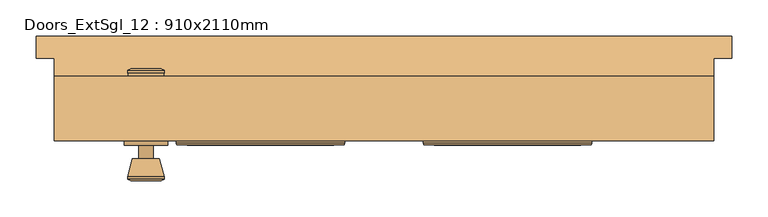
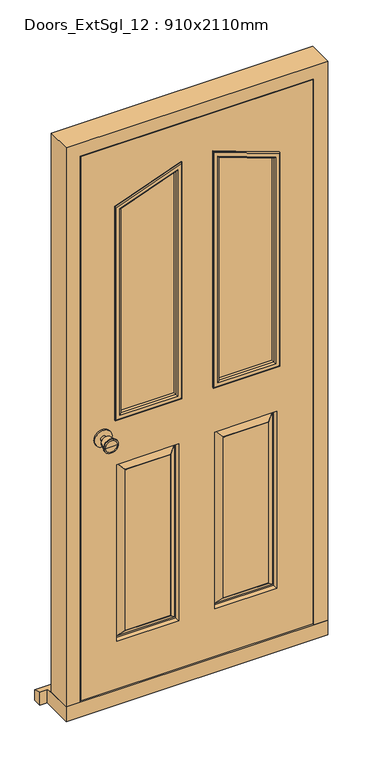
"""IFC4 building model written with IfcOpenShell, lengths in millimetres: door geometry, Doors_ExtSgl_12 : 910x2110mm."""

from ifc_helpers import new_model, si_unit, point, frame, frame_2d, origin, place, context, project, spatial, polyline, circle_curve, ellipse_curve, trimmed, segment, composite_curve, outline, extrude, faceted_brep, source, transform, mapped, element, save
from ifc_brep_helpers import plane_surface, cylinder_surface, revolved_surface, advanced_brep


def doors_extsgl_12_910x2110mm_9a09825e(model_context):
    return source(origin(), model_context, "Body", "SolidModel", [
        advanced_brep(
        [(-328.5, -18.4, 1000.0), (-318.5, -18.4, 1000.0), (-338.5, -18.4, 1000.0), (-308.0241324, -67.4, 1000.0), (-328.5, -67.4, 1000.0), (-348.9758676, -67.4, 1000.0), (-303.5, -65.5721319, 1000.0), (-353.5, -65.5721319, 1000.0), (-303.5, -62.1084537, 1000.0), (-353.5, -62.1084537, 1000.0), (-309.863764, -37.4, 1000.0), (-347.136236, -37.4, 1000.0), (-318.5, -37.4, 1000.0), (-338.5, -37.4, 1000.0)],
        [
            (0, 1),
            (1, 2, circle_curve(frame((-328.5, -18.4, 1000.0), z_axis=(0.0, 1.0, 0.0), x_axis=(-1.0, 0.0, 0.0)), 10.0)),
            (2, 0),
            (2, 1, circle_curve(frame((-328.5, -18.4, 1000.0), z_axis=(0.0, 1.0, 0.0), x_axis=(-1.0, 0.0, 0.0)), 10.0)),
            (3, 4),
            (4, 5),
            (5, 3, circle_curve(frame((-328.5, -67.4, 1000.0), z_axis=(0.0, -1.0, 0.0), x_axis=(-1.0, 0.0, 0.0)), 20.4758676)),
            (3, 5, circle_curve(frame((-328.5, -67.4, 1000.0), z_axis=(0.0, -1.0, 0.0), x_axis=(-1.0, 0.0, 0.0)), 20.4758676)),
            (6, 3),
            (5, 7),
            (7, 6, circle_curve(frame((-328.5, -65.5721319, 1000.0), z_axis=(0.0, -1.0, 0.0), x_axis=(-1.0, 0.0, 0.0)), 25.0)),
            (6, 7, circle_curve(frame((-328.5, -65.5721319, 1000.0), z_axis=(0.0, -1.0, 0.0), x_axis=(-1.0, 0.0, 0.0)), 25.0)),
            (8, 6),
            (7, 9),
            (9, 8, circle_curve(frame((-328.5, -62.1084537, 1000.0), z_axis=(0.0, -1.0, 0.0), x_axis=(-1.0, 0.0, 0.0)), 25.0)),
            (8, 9, circle_curve(frame((-328.5, -62.1084537, 1000.0), z_axis=(0.0, -1.0, 0.0), x_axis=(-1.0, 0.0, 0.0)), 25.0)),
            (10, 8),
            (9, 11),
            (11, 10, circle_curve(frame((-328.5, -37.4, 1000.0), z_axis=(0.0, -1.0, 0.0), x_axis=(-1.0, 0.0, 0.0)), 18.636236)),
            (10, 11, circle_curve(frame((-328.5, -37.4, 1000.0), z_axis=(0.0, -1.0, 0.0), x_axis=(-1.0, 0.0, 0.0)), 18.636236)),
            (12, 10),
            (11, 13),
            (13, 12, circle_curve(frame((-328.5, -37.4, 1000.0), z_axis=(0.0, -1.0, 0.0), x_axis=(-1.0, 0.0, 0.0)), 10.0)),
            (12, 13, circle_curve(frame((-328.5, -37.4, 1000.0), z_axis=(0.0, -1.0, 0.0), x_axis=(-1.0, 0.0, 0.0)), 10.0)),
            (1, 12),
            (13, 2),
        ],
        [
            plane_surface(frame((-328.5, -18.4, 1000.0), z_axis=(0.0, 1.0, 0.0), x_axis=(-1.0, 0.0, 0.0))),
            plane_surface(frame((-328.5, -67.4, 1000.0), z_axis=(0.0, -1.0, 0.0), x_axis=(-1.0, 0.0, 0.0))),
            revolved_surface(polyline([(-348.9758676, -67.4, 1000.0), (-353.5, -65.5721319, 1000.0)]), (-328.5, -18.4, 1000.0), (0.0, 1.0, 0.0)),
            cylinder_surface(frame((-328.5, -18.4, 1000.0), z_axis=(0.0, 1.0, 0.0), x_axis=(-1.0, 0.0, 0.0)), 25.0),
            revolved_surface(polyline([(-353.5, -62.1084537, 1000.0), (-347.136236, -37.4, 1000.0)]), (-328.5, -18.4, 1000.0), (0.0, 1.0, 0.0)),
            plane_surface(frame((-328.5, -37.4, 1000.0), z_axis=(0.0, 1.0, 0.0), x_axis=(-1.0, 0.0, 0.0))),
            cylinder_surface(frame((-328.5, -18.4, 1000.0), z_axis=(0.0, 1.0, 0.0), x_axis=(-1.0, 0.0, 0.0)), 10.0),
        ],
        [
            (0, [[1, 2, 3]]),
            (0, [[-3, 4, -1]]),
            (1, [[5, 6, 7]]),
            (1, [[-6, -5, 8]]),
            (2, [[9, -7, 10, 11]]),
            (2, [[-10, -8, -9, 12]]),
            (3, [[13, -11, 14, 15]]),
            (3, [[-14, -12, -13, 16]]),
            (4, [[17, -15, 18, 19]]),
            (4, [[-18, -16, -17, 20]]),
            (5, [[21, -19, 22, 23]]),
            (5, [[-22, -20, -21, 24]]),
            (6, [[25, -23, 26, -2]]),
            (6, [[-26, -24, -25, -4]]),
        ],
    ),
        extrude(outline(composite_curve([segment(trimmed(circle_curve(frame_2d((1000.0, -328.5)), 30.0), [point((1000.0, -358.5))], [point((1000.0, -298.5))], False, "CARTESIAN"), True, "CONTINUOUS"), segment(trimmed(circle_curve(frame_2d((1000.0, -328.5)), 30.0), [point((1000.0, -298.5))], [point((1000.0, -358.5))], False, "CARTESIAN"), True, "CONTINUOUS")], self_intersect=False)), frame((0.0, -18.4, 0.0), z_axis=(0.0, 1.0, 0.0), x_axis=(0.0, 0.0, 1.0)), (0.0, 0.0, 1.0), 6.0),
        advanced_brep(
        [(-328.5, 37.6, 1000.0), (-338.5, 37.6, 1000.0), (-318.5, 37.6, 1000.0), (-308.0241324, 86.6, 1000.0), (-348.9758676, 86.6, 1000.0), (-328.5, 86.6, 1000.0), (-303.5, 84.7721319, 1000.0), (-353.5, 84.7721319, 1000.0), (-303.5, 81.3084537, 1000.0), (-353.5, 81.3084537, 1000.0), (-309.863764, 56.6, 1000.0), (-347.136236, 56.6, 1000.0), (-318.5, 56.6, 1000.0), (-338.5, 56.6, 1000.0)],
        [
            (0, 1),
            (1, 2, circle_curve(frame((-328.5, 37.6, 1000.0), z_axis=(0.0, -1.0, 0.0), x_axis=(-1.0, 0.0, 0.0)), 10.0)),
            (2, 0),
            (2, 1, circle_curve(frame((-328.5, 37.6, 1000.0), z_axis=(0.0, -1.0, 0.0), x_axis=(-1.0, 0.0, 0.0)), 10.0)),
            (3, 4, circle_curve(frame((-328.5, 86.6, 1000.0), z_axis=(0.0, 1.0, 0.0), x_axis=(-1.0, 0.0, 0.0)), 20.4758676)),
            (4, 5),
            (5, 3),
            (4, 3, circle_curve(frame((-328.5, 86.6, 1000.0), z_axis=(0.0, 1.0, 0.0), x_axis=(-1.0, 0.0, 0.0)), 20.4758676)),
            (6, 7, circle_curve(frame((-328.5, 84.7721319, 1000.0), z_axis=(0.0, 1.0, 0.0), x_axis=(-1.0, 0.0, 0.0)), 25.0)),
            (7, 4),
            (3, 6),
            (7, 6, circle_curve(frame((-328.5, 84.7721319, 1000.0), z_axis=(0.0, 1.0, 0.0), x_axis=(-1.0, 0.0, 0.0)), 25.0)),
            (8, 9, circle_curve(frame((-328.5, 81.3084537, 1000.0), z_axis=(0.0, 1.0, 0.0), x_axis=(-1.0, 0.0, 0.0)), 25.0)),
            (9, 7),
            (6, 8),
            (9, 8, circle_curve(frame((-328.5, 81.3084537, 1000.0), z_axis=(0.0, 1.0, 0.0), x_axis=(-1.0, 0.0, 0.0)), 25.0)),
            (10, 11, circle_curve(frame((-328.5, 56.6, 1000.0), z_axis=(0.0, 1.0, 0.0), x_axis=(-1.0, 0.0, 0.0)), 18.636236)),
            (11, 9),
            (8, 10),
            (11, 10, circle_curve(frame((-328.5, 56.6, 1000.0), z_axis=(0.0, 1.0, 0.0), x_axis=(-1.0, 0.0, 0.0)), 18.636236)),
            (12, 13, circle_curve(frame((-328.5, 56.6, 1000.0), z_axis=(0.0, 1.0, 0.0), x_axis=(-1.0, 0.0, 0.0)), 10.0)),
            (13, 11),
            (10, 12),
            (13, 12, circle_curve(frame((-328.5, 56.6, 1000.0), z_axis=(0.0, 1.0, 0.0), x_axis=(-1.0, 0.0, 0.0)), 10.0)),
            (1, 13),
            (12, 2),
        ],
        [
            plane_surface(frame((-328.5, 37.6, 1000.0), z_axis=(0.0, -1.0, 0.0), x_axis=(-1.0, 0.0, 0.0))),
            plane_surface(frame((-328.5, 86.6, 1000.0), z_axis=(0.0, 1.0, 0.0), x_axis=(-1.0, 0.0, 0.0))),
            revolved_surface(polyline([(-348.9758676, 86.6, 1000.0), (-353.5, 84.7721319, 1000.0)]), (-328.5, 37.6, 1000.0), (0.0, -1.0, 0.0)),
            cylinder_surface(frame((-328.5, 37.6, 1000.0), z_axis=(0.0, -1.0, 0.0), x_axis=(-1.0, 0.0, 0.0)), 25.0),
            revolved_surface(polyline([(-353.5, 81.3084537, 1000.0), (-347.136236, 56.6, 1000.0)]), (-328.5, 37.6, 1000.0), (0.0, -1.0, 0.0)),
            plane_surface(frame((-328.5, 56.6, 1000.0), z_axis=(0.0, -1.0, 0.0), x_axis=(-1.0, 0.0, 0.0))),
            cylinder_surface(frame((-328.5, 37.6, 1000.0), z_axis=(0.0, -1.0, 0.0), x_axis=(-1.0, 0.0, 0.0)), 10.0),
        ],
        [
            (0, [[1, 2, 3]]),
            (0, [[-3, 4, -1]]),
            (1, [[5, 6, 7]]),
            (1, [[8, -7, -6]]),
            (2, [[9, 10, -5, 11]]),
            (2, [[12, -11, -8, -10]]),
            (3, [[13, 14, -9, 15]]),
            (3, [[16, -15, -12, -14]]),
            (4, [[17, 18, -13, 19]]),
            (4, [[20, -19, -16, -18]]),
            (5, [[21, 22, -17, 23]]),
            (5, [[24, -23, -20, -22]]),
            (6, [[-2, 25, -21, 26]]),
            (6, [[-4, -26, -24, -25]]),
        ],
    ),
        extrude(outline(composite_curve([segment(trimmed(circle_curve(frame_2d((1000.0, -328.5)), 30.0), [point((1000.0, -358.5))], [point((1000.0, -298.5))], False, "CARTESIAN"), True, "CONTINUOUS"), segment(trimmed(circle_curve(frame_2d((1000.0, -328.5)), 30.0), [point((1000.0, -298.5))], [point((1000.0, -358.5))], False, "CARTESIAN"), True, "CONTINUOUS")], self_intersect=False)), frame((0.0, 31.6, 0.0), z_axis=(0.0, 1.0, 0.0), x_axis=(0.0, 0.0, 1.0)), (0.0, 0.0, 1.0), 6.0),
        faceted_brep([(384.5, 76.6, 54.5), (455.0, 76.6, 54.5), (455.0, -12.4, 54.5), (406.5, -12.4, 54.5), (406.5, 34.6, 54.5), (384.5, 34.6, 54.5), (384.5, 76.6, 2039.5), (-384.5, 76.6, 2039.5), (-384.5, 76.6, 54.5), (-455.0, 76.6, 54.5), (-455.0, 76.6, 2110.0), (455.0, 76.6, 2110.0), (455.0, -12.4, 2110.0), (-455.0, -12.4, 2110.0), (-455.0, -12.4, 54.5), (-406.5, -12.4, 54.5), (-406.5, -12.4, 2061.5), (406.5, -12.4, 2061.5), (406.5, 34.6, 2061.5), (-406.5, 34.6, 2061.5), (-406.5, 34.6, 54.5), (-384.5, 34.6, 54.5), (-384.5, 34.6, 2039.5), (384.5, 34.6, 2039.5)], [[[0, 1, 2, 3, 4, 5]], [[1, 0, 6, 7, 8, 9, 10, 11]], [[2, 1, 11, 12]], [[3, 2, 12, 13, 14, 15, 16, 17]], [[4, 3, 17, 18]], [[5, 4, 18, 19, 20, 21, 22, 23]], [[0, 5, 23, 6]], [[8, 7, 22, 21]], [[9, 8, 21, 20, 15, 14]], [[10, 9, 14, 13]], [[16, 15, 20, 19]], [[11, 10, 13, 12]], [[17, 16, 19, 18]], [[7, 6, 23, 22]]]),
        faceted_brep([(403.5, -12.4, 58.5), (403.5, -12.4, 2058.5), (-404.4250294, -12.4, 2058.5), (-404.4250294, -12.4, 58.5), (62.5, -12.4, 1058.5), (62.5, -12.4, 1908.5), (278.5, -12.4, 1829.8824294), (278.5, -12.4, 1058.5), (-278.5, -12.4, 1058.5), (-278.5, -12.4, 1829.8824294), (-62.5, -12.4, 1908.5), (-62.5, -12.4, 1058.5), (-62.5, -12.4, 883.5), (-62.5, -12.4, 233.5), (-278.5, -12.4, 233.5), (-278.5, -12.4, 883.5), (278.5, -12.4, 883.5), (278.5, -12.4, 233.5), (62.5, -12.4, 233.5), (62.5, -12.4, 883.5), (-92.5, -12.4, 263.5), (-92.5, -12.4, 853.5), (-248.5, -12.4, 853.5), (-248.5, -12.4, 263.5), (248.5, -12.4, 263.5), (248.5, -12.4, 853.5), (92.5, -12.4, 853.5), (92.5, -12.4, 263.5), (403.5, 31.6, 58.5), (-404.4250294, 31.6, 58.5), (-404.4250294, 31.6, 2058.5), (403.5, 31.6, 2058.5), (62.5, 31.6, 1058.5), (278.5, 31.6, 1058.5), (278.5, 31.6, 1829.8824294), (62.5, 31.6, 1908.5), (-278.5, 31.6, 1058.5), (-62.5, 31.6, 1058.5), (-62.5, 31.6, 1908.5), (-278.5, 31.6, 1829.8824294), (62.5, 31.6, 883.5), (62.5, 31.6, 233.5), (278.5, 31.6, 233.5), (278.5, 31.6, 883.5), (-278.5, 31.6, 883.5), (-278.5, 31.6, 233.5), (-62.5, 31.6, 233.5), (-62.5, 31.6, 883.5), (92.5, 31.6, 263.5), (92.5, 31.6, 853.5), (248.5, 31.6, 853.5), (248.5, 31.6, 263.5), (-248.5, 31.6, 263.5), (-248.5, 31.6, 853.5), (-92.5, 31.6, 853.5), (-92.5, 31.6, 263.5), (65.5, 16.6, 880.5), (65.5, 16.6, 236.5), (90.5, 30.6, 855.5), (90.5, 30.6, 261.5), (70.5, 16.6, 241.5), (70.5, 16.6, 875.5), (92.5, 30.6, 263.5), (92.5, 30.6, 853.5), (275.5, 16.6, 236.5), (250.5, 30.6, 261.5), (270.5, 16.6, 241.5), (248.5, 30.6, 263.5), (275.5, 16.6, 880.5), (250.5, 30.6, 855.5), (270.5, 16.6, 875.5), (248.5, 30.6, 853.5), (-275.5, 16.6, 880.5), (-275.5, 16.6, 236.5), (-250.5, 30.6, 855.5), (-250.5, 30.6, 261.5), (-270.5, 16.6, 241.5), (-270.5, 16.6, 875.5), (-248.5, 30.6, 263.5), (-248.5, 30.6, 853.5), (-65.5, 16.6, 236.5), (-90.5, 30.6, 261.5), (-70.5, 16.6, 241.5), (-92.5, 30.6, 263.5), (-65.5, 16.6, 880.5), (-90.5, 30.6, 855.5), (-70.5, 16.6, 875.5), (-92.5, 30.6, 853.5), (-92.5, -11.4, 263.5), (-92.5, -11.4, 853.5), (-70.5, 2.6, 241.5), (-70.5, 2.6, 875.5), (-90.5, -11.4, 855.5), (-90.5, -11.4, 261.5), (-65.5, 2.6, 880.5), (-65.5, 2.6, 236.5), (-248.5, -11.4, 853.5), (-270.5, 2.6, 875.5), (-250.5, -11.4, 855.5), (-275.5, 2.6, 880.5), (-248.5, -11.4, 263.5), (-270.5, 2.6, 241.5), (-250.5, -11.4, 261.5), (-275.5, 2.6, 236.5), (275.5, 2.6, 880.5), (275.5, 2.6, 236.5), (250.5, -11.4, 855.5), (250.5, -11.4, 261.5), (270.5, 2.6, 241.5), (270.5, 2.6, 875.5), (248.5, -11.4, 263.5), (248.5, -11.4, 853.5), (65.5, 2.6, 236.5), (90.5, -11.4, 261.5), (70.5, 2.6, 241.5), (92.5, -11.4, 263.5), (65.5, 2.6, 880.5), (90.5, -11.4, 855.5), (70.5, 2.6, 875.5), (92.5, -11.4, 853.5)], [[[0, 1, 2, 3], [4, 5, 6, 7], [8, 9, 10, 11], [12, 13, 14, 15], [16, 17, 18, 19]], [[20, 21, 22, 23]], [[24, 25, 26, 27]], [[28, 29, 30, 31], [32, 33, 34, 35], [36, 37, 38, 39], [40, 41, 42, 43], [44, 45, 46, 47]], [[48, 49, 50, 51]], [[52, 53, 54, 55]], [[1, 0, 28, 31]], [[2, 1, 31, 30]], [[3, 2, 30, 29]], [[0, 3, 29, 28]], [[5, 4, 32, 35]], [[6, 5, 35, 34]], [[7, 6, 34, 33]], [[4, 7, 33, 32]], [[9, 8, 36, 39]], [[10, 9, 39, 38]], [[11, 10, 38, 37]], [[8, 11, 37, 36]], [[56, 57, 41, 40]], [[58, 59, 60, 61]], [[48, 62, 63, 49]], [[41, 57, 64, 42]], [[60, 59, 65, 66]], [[62, 48, 51, 67]], [[42, 64, 68, 43]], [[66, 65, 69, 70]], [[67, 51, 50, 71]], [[56, 40, 43, 68]], [[57, 56, 68, 64], [61, 60, 66, 70]], [[58, 61, 70, 69]], [[59, 58, 69, 65], [63, 62, 67, 71]], [[49, 63, 71, 50]], [[72, 73, 45, 44]], [[74, 75, 76, 77]], [[52, 78, 79, 53]], [[45, 73, 80, 46]], [[76, 75, 81, 82]], [[78, 52, 55, 83]], [[46, 80, 84, 47]], [[82, 81, 85, 86]], [[83, 55, 54, 87]], [[72, 44, 47, 84]], [[73, 72, 84, 80], [77, 76, 82, 86]], [[74, 77, 86, 85]], [[75, 74, 85, 81], [79, 78, 83, 87]], [[53, 79, 87, 54]], [[88, 89, 21, 20]], [[90, 91, 92, 93]], [[12, 94, 95, 13]], [[21, 89, 96, 22]], [[92, 91, 97, 98]], [[94, 12, 15, 99]], [[22, 96, 100, 23]], [[98, 97, 101, 102]], [[99, 15, 14, 103]], [[88, 20, 23, 100]], [[93, 92, 98, 102], [89, 88, 100, 96]], [[90, 93, 102, 101]], [[95, 94, 99, 103], [91, 90, 101, 97]], [[13, 95, 103, 14]], [[104, 105, 17, 16]], [[106, 107, 108, 109]], [[24, 110, 111, 25]], [[17, 105, 112, 18]], [[108, 107, 113, 114]], [[110, 24, 27, 115]], [[18, 112, 116, 19]], [[114, 113, 117, 118]], [[115, 27, 26, 119]], [[104, 16, 19, 116]], [[105, 104, 116, 112], [109, 108, 114, 118]], [[106, 109, 118, 117]], [[107, 106, 117, 113], [111, 110, 115, 119]], [[25, 111, 119, 26]]]),
        faceted_brep([(480.0, 131.6, 0.0), (480.0, 131.6, 38.5947221), (480.0, 101.6, 47.2703282), (480.0, 101.6, 0.0), (-480.0, 131.6, 38.5947221), (-480.0, 131.6, 0.0), (-480.0, 101.6, 0.0), (-480.0, 101.6, 47.2703282), (455.0, 101.6, 0.0), (455.0, -12.4, 0.0), (-455.0, -12.4, 0.0), (-455.0, 101.6, 0.0), (-455.0, 101.6, 47.2703282), (-455.0, 76.6, 54.5), (455.0, 76.6, 54.5), (455.0, 101.6, 47.2703282), (-455.0, -12.4, 54.5), (455.0, -12.4, 54.5)], [[[0, 1, 2, 3]], [[4, 5, 6, 7]], [[5, 0, 3, 8, 9, 10, 11, 6]], [[1, 0, 5, 4]], [[1, 4, 7, 12, 13, 14, 15, 2]], [[13, 16, 17, 14]], [[16, 10, 9, 17]], [[12, 11, 10, 16, 13]], [[11, 12, 7, 6]], [[8, 15, 14, 17, 9]], [[15, 8, 3, 2]]]),
        extrude(outline(polyline([(1058.5, 278.5), (1829.8824294, 278.5), (1908.5, 62.5), (1058.5, 62.5), (1058.5, 278.5)])), frame((0.0, -2.4, 0.0), z_axis=(0.0, 1.0, 0.0), x_axis=(0.0, 0.0, 1.0)), (0.0, 0.0, 1.0), 24.0),
        extrude(outline(polyline([(1058.5, -62.5), (1908.5, -62.5), (1829.8824294, -278.5), (1058.5, -278.5), (1058.5, -62.5)])), frame((0.0, -2.4, 0.0), z_axis=(0.0, 1.0, 0.0), x_axis=(0.0, 0.0, 1.0)), (0.0, 0.0, 1.0), 24.0),
        advanced_brep(
        [(286.5, 35.6, 1835.4840897), (286.5, 31.6, 1835.4840897), (286.5, 31.6, 1050.5), (286.5, 35.6, 1050.5), (284.5, 37.6, 1834.0836746), (284.5, 37.6, 1052.5), (266.5, 32.6, 1821.4799389), (271.5, 37.6, 1824.9809766), (271.5, 37.6, 1065.5), (266.5, 32.6, 1070.5), (266.5, 21.6, 1821.4799389), (266.5, 21.6, 1070.5), (278.5, 31.6, 1829.8824294), (278.5, 21.6, 1829.8824294), (278.5, 21.6, 1058.5), (278.5, 31.6, 1058.5), (54.5, 31.6, 1050.5), (54.5, 35.6, 1050.5), (56.5, 37.6, 1052.5), (69.5, 37.6, 1065.5), (74.5, 32.6, 1070.5), (74.5, 21.6, 1070.5), (62.5, 21.6, 1058.5), (62.5, 31.6, 1058.5), (54.5, 31.6, 1919.9251841), (54.5, 35.6, 1919.9251841), (56.5, 37.6, 1917.068888), (69.5, 37.6, 1898.502964), (74.5, 32.6, 1891.3622239), (74.5, 21.6, 1891.3622239), (62.5, 21.6, 1908.5), (62.5, 31.6, 1908.5)],
        [
            (0, 1),
            (1, 2),
            (2, 3),
            (3, 0),
            (4, 0, ellipse_curve(frame((284.5, 35.6, 1834.0836746), z_axis=(0.5735764363510463, 0.0, -0.8191520442889918), x_axis=(0.8191520442889918, 0.0, 0.5735764363510459)), 2.4415492, 2.0)),
            (3, 5, ellipse_curve(frame((284.5, 35.6, 1052.5), z_axis=(0.7071067811865475, 0.0, 0.7071067811865475), x_axis=(-0.7071067811865474, 0.0, 0.7071067811865476)), 2.8284271, 2.0)),
            (5, 4),
            (6, 7, ellipse_curve(frame((271.5, 32.6, 1824.9809766), z_axis=(0.5735764363510463, 0.0, -0.8191520442889918), x_axis=(0.8191520442889918, 0.0, 0.5735764363510459)), 6.1038729, 5.0)),
            (7, 8),
            (8, 9, ellipse_curve(frame((271.5, 32.6, 1065.5), z_axis=(0.7071067811865475, 0.0, 0.7071067811865475), x_axis=(-0.7071067811865474, 0.0, 0.7071067811865476)), 7.0710678, 5.0)),
            (9, 6),
            (10, 6),
            (9, 11),
            (11, 10),
            (12, 13),
            (13, 14),
            (14, 15),
            (15, 12),
            (2, 16),
            (16, 17),
            (17, 3),
            (17, 18, ellipse_curve(frame((56.5, 35.6, 1052.5), z_axis=(0.7071067811865475, 0.0, -0.7071067811865475), x_axis=(0.7071067811865476, 0.0, 0.7071067811865474)), 2.8284271, 2.0)),
            (18, 5),
            (8, 19),
            (19, 20, ellipse_curve(frame((69.5, 32.6, 1065.5), z_axis=(0.7071067811865475, 0.0, -0.7071067811865475), x_axis=(0.7071067811865476, 0.0, 0.7071067811865474)), 7.0710678, 5.0)),
            (20, 9),
            (20, 21),
            (21, 11),
            (14, 22),
            (22, 23),
            (23, 15),
            (16, 24),
            (24, 25),
            (25, 17),
            (25, 26, ellipse_curve(frame((56.5, 35.6, 1917.068888), z_axis=(-0.8191520442889917, 0.0, -0.5735764363510462), x_axis=(0.5735764363510462, 0.0, -0.8191520442889918)), 3.4868936, 2.0)),
            (26, 18),
            (19, 27),
            (27, 28, ellipse_curve(frame((69.5, 32.6, 1898.502964), z_axis=(-0.8191520442889917, 0.0, -0.5735764363510462), x_axis=(0.5735764363510462, 0.0, -0.8191520442889918)), 8.717234, 5.0)),
            (28, 20),
            (28, 29),
            (29, 21),
            (22, 30),
            (30, 31),
            (31, 23),
            (24, 1),
            (0, 25),
            (4, 26),
            (7, 27),
            (6, 28),
            (10, 29),
            (13, 30),
            (12, 31),
        ],
        [
            plane_surface(frame((286.5, 31.6, 1835.4840897), z_axis=(1.0, 0.0, 0.0), x_axis=(0.0, 0.0, -1.0))),
            cylinder_surface(frame((284.5, 35.6, 1829.8824294), z_axis=(0.0, 0.0, 1.0), x_axis=(1.0, 0.0, 0.0)), 2.0),
            cylinder_surface(frame((271.5, 32.6, 1829.8824294), z_axis=(0.0, 0.0, 1.0), x_axis=(1.0, 0.0, 0.0)), 5.0),
            plane_surface(frame((266.5, 32.6, 1821.4799389), z_axis=(-1.0, 0.0, 0.0), x_axis=(0.0, 0.0, -1.0))),
            plane_surface(frame((278.5, 21.6, 1829.8824294), z_axis=(1.0, 0.0, 0.0), x_axis=(0.0, 0.0, -1.0))),
            plane_surface(frame((286.5, 31.6, 1050.5), z_axis=(0.0, 0.0, -1.0), x_axis=(-1.0, 0.0, 0.0))),
            cylinder_surface(frame((278.5, 35.6, 1052.5), z_axis=(1.0, 0.0, 0.0), x_axis=(0.0, 0.0, -1.0)), 2.0),
            cylinder_surface(frame((278.5, 32.6, 1065.5), z_axis=(1.0, 0.0, 0.0), x_axis=(0.0, 0.0, -1.0)), 5.0),
            plane_surface(frame((266.5, 32.6, 1070.5), z_axis=(0.0, 0.0, 1.0), x_axis=(-1.0, 0.0, 0.0))),
            plane_surface(frame((278.5, 21.6, 1058.5), z_axis=(0.0, 0.0, -1.0), x_axis=(-1.0, 0.0, 0.0))),
            plane_surface(frame((54.5, 31.6, 1050.5), z_axis=(-1.0, 0.0, 0.0), x_axis=(0.0, 0.0, 1.0))),
            cylinder_surface(frame((56.5, 35.6, 1058.5), z_axis=(0.0, 0.0, -1.0), x_axis=(-1.0, 0.0, 0.0)), 2.0),
            cylinder_surface(frame((69.5, 32.6, 1058.5), z_axis=(0.0, 0.0, -1.0), x_axis=(-1.0, 0.0, 0.0)), 5.0),
            plane_surface(frame((74.5, 32.6, 1070.5), z_axis=(1.0, 0.0, 0.0), x_axis=(0.0, 0.0, 1.0))),
            plane_surface(frame((62.5, 21.6, 1058.5), z_axis=(-1.0, 0.0, 0.0), x_axis=(0.0, 0.0, 1.0))),
            plane_surface(frame((54.5, 31.6, 1919.9251841), z_axis=(0.3420201433256683, 0.0, 0.9396926207859085), x_axis=(0.9396926207859085, 0.0, -0.3420201433256683))),
            cylinder_surface(frame((64.5521209, 35.6, 1914.1381557), z_axis=(-0.9396926207859085, 0.0, 0.34202014332566844), x_axis=(0.34202014332566844, 0.0, 0.9396926207859085)), 2.0),
            plane_surface(frame((56.5, 37.6, 1917.068888), z_axis=(0.0, 1.0, 0.0), x_axis=(0.9396926207859085, 0.0, -0.34202014332566844))),
            cylinder_surface(frame((60.105859, 32.6, 1901.9221517), z_axis=(-0.9396926207859085, 0.0, 0.34202014332566844), x_axis=(0.34202014332566844, 0.0, 0.9396926207859085)), 5.0),
            plane_surface(frame((74.5, 32.6, 1891.3622239), z_axis=(-0.34202014332566844, 0.0, -0.9396926207859085), x_axis=(0.9396926207859085, 0.0, -0.34202014332566844))),
            plane_surface(frame((74.5, 21.6, 1891.3622239), z_axis=(0.0, -1.0, 0.0), x_axis=(0.9396926207859088, 0.0, -0.3420201433256677))),
            plane_surface(frame((62.5, 21.6, 1908.5), z_axis=(0.34202014332566905, 0.0, 0.9396926207859083), x_axis=(0.9396926207859083, 0.0, -0.34202014332566905))),
            plane_surface(frame((62.5, 31.6, 1908.5), z_axis=(0.0, -1.0, 0.0), x_axis=(0.9396926207859083, 0.0, -0.3420201433256691))),
        ],
        [
            (0, [[1, 2, 3, 4]]),
            (1, [[5, -4, 6, 7]]),
            (2, [[8, 9, 10, 11]]),
            (3, [[12, -11, 13, 14]]),
            (4, [[15, 16, 17, 18]]),
            (5, [[-3, 19, 20, 21]]),
            (6, [[-6, -21, 22, 23]]),
            (7, [[-10, 24, 25, 26]]),
            (8, [[-13, -26, 27, 28]]),
            (9, [[-17, 29, 30, 31]]),
            (10, [[-20, 32, 33, 34]]),
            (11, [[-22, -34, 35, 36]]),
            (12, [[-25, 37, 38, 39]]),
            (13, [[-27, -39, 40, 41]]),
            (14, [[-30, 42, 43, 44]]),
            (15, [[-33, 45, -1, 46]]),
            (16, [[-35, -46, -5, 47]]),
            (17, [[-23, -36, -47, -7], [48, -37, -24, -9]]),
            (18, [[-38, -48, -8, 49]]),
            (19, [[-40, -49, -12, 50]]),
            (20, [[51, -42, -29, -16], [-28, -41, -50, -14]]),
            (21, [[-43, -51, -15, 52]]),
            (22, [[-45, -32, -19, -2], [-31, -44, -52, -18]]),
        ],
    ),
        advanced_brep(
        [(-54.5, 35.6, 1050.5), (-54.5, 31.6, 1050.5), (-286.5, 31.6, 1050.5), (-286.5, 35.6, 1050.5), (-56.5, 37.6, 1052.5), (-284.5, 37.6, 1052.5), (-74.5, 32.6, 1070.5), (-69.5, 37.6, 1065.5), (-271.5, 37.6, 1065.5), (-266.5, 32.6, 1070.5), (-74.5, 21.6, 1070.5), (-266.5, 21.6, 1070.5), (-62.5, 31.6, 1058.5), (-62.5, 21.6, 1058.5), (-278.5, 21.6, 1058.5), (-278.5, 31.6, 1058.5), (-286.5, 31.6, 1835.4840897), (-286.5, 35.6, 1835.4840897), (-284.5, 37.6, 1834.0836746), (-271.5, 37.6, 1824.9809766), (-266.5, 32.6, 1821.4799389), (-266.5, 21.6, 1821.4799389), (-278.5, 21.6, 1829.8824294), (-278.5, 31.6, 1829.8824294), (-54.5, 31.6, 1919.9251841), (-54.5, 35.6, 1919.9251841), (-56.5, 37.6, 1917.068888), (-69.5, 37.6, 1898.502964), (-74.5, 32.6, 1891.3622239), (-74.5, 21.6, 1891.3622239), (-62.5, 21.6, 1908.5), (-62.5, 31.6, 1908.5)],
        [
            (0, 1),
            (1, 2),
            (2, 3),
            (3, 0),
            (4, 0, ellipse_curve(frame((-56.5, 35.6, 1052.5), z_axis=(-0.7071067811865475, 0.0, -0.7071067811865475), x_axis=(0.7071067811865476, 0.0, -0.7071067811865475)), 2.8284271, 2.0)),
            (3, 5, ellipse_curve(frame((-284.5, 35.6, 1052.5), z_axis=(0.7071067811865476, 0.0, -0.7071067811865475), x_axis=(0.7071067811865475, 0.0, 0.7071067811865475)), 2.8284271, 2.0)),
            (5, 4),
            (6, 7, ellipse_curve(frame((-69.5, 32.6, 1065.5), z_axis=(-0.7071067811865475, 0.0, -0.7071067811865475), x_axis=(0.7071067811865476, 0.0, -0.7071067811865475)), 7.0710678, 5.0)),
            (7, 8),
            (8, 9, ellipse_curve(frame((-271.5, 32.6, 1065.5), z_axis=(0.7071067811865476, 0.0, -0.7071067811865475), x_axis=(0.7071067811865475, 0.0, 0.7071067811865475)), 7.0710678, 5.0)),
            (9, 6),
            (10, 6),
            (9, 11),
            (11, 10),
            (12, 13),
            (13, 14),
            (14, 15),
            (15, 12),
            (2, 16),
            (16, 17),
            (17, 3),
            (17, 18, ellipse_curve(frame((-284.5, 35.6, 1834.0836746), z_axis=(-0.5735764363510245, 0.0, -0.8191520442890069), x_axis=(0.8191520442890068, 0.0, -0.5735764363510246)), 2.4415492, 2.0)),
            (18, 5),
            (8, 19),
            (19, 20, ellipse_curve(frame((-271.5, 32.6, 1824.9809766), z_axis=(-0.5735764363510245, 0.0, -0.8191520442890069), x_axis=(0.8191520442890068, 0.0, -0.5735764363510246)), 6.1038729, 5.0)),
            (20, 9),
            (20, 21),
            (21, 11),
            (14, 22),
            (22, 23),
            (23, 15),
            (16, 24),
            (24, 25),
            (25, 17),
            (25, 26, ellipse_curve(frame((-56.5, 35.6, 1917.068888), z_axis=(-0.8191520442890069, 0.0, 0.5735764363510246), x_axis=(-0.5735764363510246, 0.0, -0.8191520442890069)), 3.4868936, 2.0)),
            (26, 18),
            (19, 27),
            (27, 28, ellipse_curve(frame((-69.5, 32.6, 1898.502964), z_axis=(-0.8191520442890069, 0.0, 0.5735764363510246), x_axis=(-0.5735764363510246, 0.0, -0.8191520442890069)), 8.717234, 5.0)),
            (28, 20),
            (28, 29),
            (29, 21),
            (22, 30),
            (30, 31),
            (31, 23),
            (24, 1),
            (0, 25),
            (4, 26),
            (7, 27),
            (6, 28),
            (10, 29),
            (13, 30),
            (12, 31),
        ],
        [
            plane_surface(frame((-54.5, 31.6, 1050.5), z_axis=(0.0, 0.0, -1.0), x_axis=(-1.0, 0.0, 0.0))),
            cylinder_surface(frame((-62.5, 35.6, 1052.5), z_axis=(1.0, 0.0, 0.0), x_axis=(0.0, 0.0, -1.0)), 2.0),
            cylinder_surface(frame((-62.5, 32.6, 1065.5), z_axis=(1.0, 0.0, 0.0), x_axis=(0.0, 0.0, -1.0)), 5.0),
            plane_surface(frame((-74.5, 32.6, 1070.5), z_axis=(0.0, 0.0, 1.0), x_axis=(-1.0, 0.0, 0.0))),
            plane_surface(frame((-62.5, 21.6, 1058.5), z_axis=(0.0, 0.0, -1.0), x_axis=(-1.0, 0.0, 0.0))),
            plane_surface(frame((-286.5, 31.6, 1050.5), z_axis=(-1.0, 0.0, 0.0), x_axis=(0.0, 0.0, 1.0))),
            cylinder_surface(frame((-284.5, 35.6, 1058.5), z_axis=(0.0, 0.0, -1.0), x_axis=(-1.0, 0.0, 0.0)), 2.0),
            cylinder_surface(frame((-271.5, 32.6, 1058.5), z_axis=(0.0, 0.0, -1.0), x_axis=(-1.0, 0.0, 0.0)), 5.0),
            plane_surface(frame((-266.5, 32.6, 1070.5), z_axis=(1.0, 0.0, 0.0), x_axis=(0.0, 0.0, 1.0))),
            plane_surface(frame((-278.5, 21.6, 1058.5), z_axis=(-1.0, 0.0, 0.0), x_axis=(0.0, 0.0, 1.0))),
            plane_surface(frame((-286.5, 31.6, 1835.4840897), z_axis=(-0.34202014332571895, 0.0, 0.9396926207858901), x_axis=(0.9396926207858901, 0.0, 0.34202014332571895))),
            cylinder_surface(frame((-280.5521209, 35.6, 1835.5205851), z_axis=(-0.9396926207858904, 0.0, -0.3420201433257182), x_axis=(-0.3420201433257182, 0.0, 0.9396926207858904)), 2.0),
            cylinder_surface(frame((-276.105859, 32.6, 1823.3045811), z_axis=(-0.9396926207858904, 0.0, -0.3420201433257182), x_axis=(-0.3420201433257182, 0.0, 0.9396926207858904)), 5.0),
            plane_surface(frame((-266.5, 32.6, 1821.4799389), z_axis=(0.3420201433257189, 0.0, -0.9396926207858901), x_axis=(0.9396926207858901, 0.0, 0.3420201433257189))),
            plane_surface(frame((-278.5, 21.6, 1829.8824294), z_axis=(-0.3420201433257181, 0.0, 0.9396926207858906), x_axis=(0.9396926207858906, 0.0, 0.3420201433257181))),
            plane_surface(frame((-54.5, 31.6, 1919.9251841), z_axis=(1.0, 0.0, 0.0), x_axis=(0.0, 0.0, -1.0))),
            cylinder_surface(frame((-56.5, 35.6, 1908.5), z_axis=(0.0, 0.0, 1.0), x_axis=(1.0, 0.0, 0.0)), 2.0),
            plane_surface(frame((-56.5, 37.6, 1917.068888), z_axis=(0.0, 1.0, 0.0), x_axis=(0.0, 0.0, -1.0))),
            cylinder_surface(frame((-69.5, 32.6, 1908.5), z_axis=(0.0, 0.0, 1.0), x_axis=(1.0, 0.0, 0.0)), 5.0),
            plane_surface(frame((-74.5, 32.6, 1891.3622239), z_axis=(-1.0, 0.0, 0.0), x_axis=(0.0, 0.0, -1.0))),
            plane_surface(frame((-74.5, 21.6, 1891.3622239), z_axis=(0.0, -1.0, 0.0), x_axis=(0.0, 0.0, -1.0))),
            plane_surface(frame((-62.5, 21.6, 1908.5), z_axis=(1.0, 0.0, 0.0), x_axis=(0.0, 0.0, -1.0))),
            plane_surface(frame((-62.5, 31.6, 1908.5), z_axis=(0.0, -1.0, 0.0), x_axis=(0.0, 0.0, -1.0))),
        ],
        [
            (0, [[1, 2, 3, 4]]),
            (1, [[5, -4, 6, 7]]),
            (2, [[8, 9, 10, 11]]),
            (3, [[12, -11, 13, 14]]),
            (4, [[15, 16, 17, 18]]),
            (5, [[-3, 19, 20, 21]]),
            (6, [[-6, -21, 22, 23]]),
            (7, [[-10, 24, 25, 26]]),
            (8, [[-13, -26, 27, 28]]),
            (9, [[-17, 29, 30, 31]]),
            (10, [[-20, 32, 33, 34]]),
            (11, [[-22, -34, 35, 36]]),
            (12, [[-25, 37, 38, 39]]),
            (13, [[-27, -39, 40, 41]]),
            (14, [[-30, 42, 43, 44]]),
            (15, [[-33, 45, -1, 46]]),
            (16, [[-35, -46, -5, 47]]),
            (17, [[-23, -36, -47, -7], [48, -37, -24, -9]]),
            (18, [[-38, -48, -8, 49]]),
            (19, [[-40, -49, -12, 50]]),
            (20, [[51, -42, -29, -16], [-28, -41, -50, -14]]),
            (21, [[-43, -51, -15, 52]]),
            (22, [[-45, -32, -19, -2], [-31, -44, -52, -18]]),
        ],
    ),
        advanced_brep(
        [(-278.5, -2.4, 1829.8824294), (-278.5, -12.4, 1829.8824294), (-62.5, -12.4, 1908.5), (-62.5, -2.4, 1908.5), (-266.5, -13.4, 1821.4799389), (-266.5, -2.4, 1821.4799389), (-74.5, -2.4, 1891.3622239), (-74.5, -13.4, 1891.3622239), (-271.5, -18.4, 1824.9809766), (-69.5, -18.4, 1898.502964), (-286.5, -16.4, 1835.4840897), (-284.5, -18.4, 1834.0836746), (-56.5, -18.4, 1917.068888), (-54.5, -16.4, 1919.9251841), (-286.5, -12.4, 1835.4840897), (-54.5, -12.4, 1919.9251841), (-62.5, -12.4, 1058.5), (-62.5, -2.4, 1058.5), (-74.5, -2.4, 1070.5), (-74.5, -13.4, 1070.5), (-69.5, -18.4, 1065.5), (-56.5, -18.4, 1052.5), (-54.5, -16.4, 1050.5), (-54.5, -12.4, 1050.5), (-278.5, -12.4, 1058.5), (-278.5, -2.4, 1058.5), (-266.5, -2.4, 1070.5), (-266.5, -13.4, 1070.5), (-271.5, -18.4, 1065.5), (-284.5, -18.4, 1052.5), (-286.5, -16.4, 1050.5), (-286.5, -12.4, 1050.5)],
        [
            (0, 1),
            (1, 2),
            (2, 3),
            (3, 0),
            (4, 5),
            (5, 6),
            (6, 7),
            (7, 4),
            (8, 4, ellipse_curve(frame((-271.5, -13.4, 1824.9809766), z_axis=(0.5735764363510244, 0.0, 0.819152044289007), x_axis=(-0.8191520442890069, 0.0, 0.5735764363510246)), 6.1038729, 5.0)),
            (7, 9, ellipse_curve(frame((-69.5, -13.4, 1898.502964), z_axis=(-0.8191520442890071, 0.0, 0.5735764363510244), x_axis=(-0.5735764363510243, 0.0, -0.8191520442890072)), 8.717234, 5.0)),
            (9, 8),
            (10, 11, ellipse_curve(frame((-284.5, -16.4, 1834.0836746), z_axis=(0.5735764363510244, 0.0, 0.819152044289007), x_axis=(-0.8191520442890069, 0.0, 0.5735764363510246)), 2.4415492, 2.0)),
            (11, 12),
            (12, 13, ellipse_curve(frame((-56.5, -16.4, 1917.068888), z_axis=(-0.8191520442890071, 0.0, 0.5735764363510244), x_axis=(-0.5735764363510243, 0.0, -0.8191520442890072)), 3.4868936, 2.0)),
            (13, 10),
            (14, 10),
            (13, 15),
            (15, 14),
            (2, 16),
            (16, 17),
            (17, 3),
            (6, 18),
            (18, 19),
            (19, 7),
            (19, 20, ellipse_curve(frame((-69.5, -13.4, 1065.5), z_axis=(0.7071067811865474, 0.0, 0.7071067811865476), x_axis=(-0.7071067811865476, 0.0, 0.7071067811865475)), 7.0710678, 5.0)),
            (20, 9),
            (12, 21),
            (21, 22, ellipse_curve(frame((-56.5, -16.4, 1052.5), z_axis=(0.7071067811865474, 0.0, 0.7071067811865476), x_axis=(-0.7071067811865476, 0.0, 0.7071067811865475)), 2.8284271, 2.0)),
            (22, 13),
            (22, 23),
            (23, 15),
            (16, 24),
            (24, 25),
            (25, 17),
            (18, 26),
            (26, 27),
            (27, 19),
            (27, 28, ellipse_curve(frame((-271.5, -13.4, 1065.5), z_axis=(0.7071067811865476, 0.0, -0.7071067811865474), x_axis=(0.7071067811865475, 0.0, 0.7071067811865475)), 7.0710678, 5.0)),
            (28, 20),
            (21, 29),
            (29, 30, ellipse_curve(frame((-284.5, -16.4, 1052.5), z_axis=(0.7071067811865476, 0.0, -0.7071067811865474), x_axis=(0.7071067811865475, 0.0, 0.7071067811865475)), 2.8284271, 2.0)),
            (30, 22),
            (30, 31),
            (31, 23),
            (31, 14),
            (1, 24),
            (0, 25),
            (5, 26),
            (4, 27),
            (8, 28),
            (11, 29),
            (10, 30),
        ],
        [
            plane_surface(frame((-278.5, -12.4, 1829.8824294), z_axis=(-0.3420201433257189, 0.0, 0.9396926207858901), x_axis=(0.9396926207858901, 0.0, 0.3420201433257189))),
            plane_surface(frame((-266.5, -2.4, 1821.4799389), z_axis=(0.34202014332571906, 0.0, -0.9396926207858901), x_axis=(0.9396926207858901, 0.0, 0.34202014332571906))),
            cylinder_surface(frame((-276.105859, -13.4, 1823.3045811), z_axis=(-0.9396926207858903, 0.0, -0.3420201433257184), x_axis=(-0.3420201433257184, 0.0, 0.9396926207858903)), 5.0),
            cylinder_surface(frame((-280.5521209, -16.4, 1835.5205851), z_axis=(-0.9396926207858903, 0.0, -0.3420201433257184), x_axis=(-0.3420201433257184, 0.0, 0.9396926207858903)), 2.0),
            plane_surface(frame((-286.5, -16.4, 1835.4840897), z_axis=(-0.3420201433257183, 0.0, 0.9396926207858904), x_axis=(0.9396926207858904, 0.0, 0.3420201433257183))),
            plane_surface(frame((-62.5, -12.4, 1908.5), z_axis=(1.0, 0.0, 0.0), x_axis=(0.0, 0.0, -1.0))),
            plane_surface(frame((-74.5, -2.4, 1891.3622239), z_axis=(-1.0, 0.0, 0.0), x_axis=(0.0, 0.0, -1.0))),
            cylinder_surface(frame((-69.5, -13.4, 1908.5), z_axis=(0.0, 0.0, 1.0), x_axis=(1.0, 0.0, 0.0)), 5.0),
            cylinder_surface(frame((-56.5, -16.4, 1908.5), z_axis=(0.0, 0.0, 1.0), x_axis=(1.0, 0.0, 0.0)), 2.0),
            plane_surface(frame((-54.5, -16.4, 1919.9251841), z_axis=(1.0, 0.0, 0.0), x_axis=(0.0, 0.0, -1.0))),
            plane_surface(frame((-62.5, -12.4, 1058.5), z_axis=(0.0, 0.0, -1.0), x_axis=(-1.0, 0.0, 0.0))),
            plane_surface(frame((-74.5, -2.4, 1070.5), z_axis=(0.0, 0.0, 1.0), x_axis=(-1.0, 0.0, 0.0))),
            cylinder_surface(frame((-62.5, -13.4, 1065.5), z_axis=(1.0, 0.0, 0.0), x_axis=(0.0, 0.0, -1.0)), 5.0),
            cylinder_surface(frame((-62.5, -16.4, 1052.5), z_axis=(1.0, 0.0, 0.0), x_axis=(0.0, 0.0, -1.0)), 2.0),
            plane_surface(frame((-54.5, -16.4, 1050.5), z_axis=(0.0, 0.0, -1.0), x_axis=(-1.0, 0.0, 0.0))),
            plane_surface(frame((-286.5, -12.4, 1050.5), z_axis=(0.0, 1.0, 0.0), x_axis=(0.0, 0.0, 1.0))),
            plane_surface(frame((-278.5, -12.4, 1058.5), z_axis=(-1.0, 0.0, 0.0), x_axis=(0.0, 0.0, 1.0))),
            plane_surface(frame((-278.5, -2.4, 1058.5), z_axis=(0.0, 1.0, 0.0), x_axis=(0.0, 0.0, 1.0))),
            plane_surface(frame((-266.5, -2.4, 1070.5), z_axis=(1.0, 0.0, 0.0), x_axis=(0.0, 0.0, 1.0))),
            cylinder_surface(frame((-271.5, -13.4, 1058.5), z_axis=(0.0, 0.0, -1.0), x_axis=(-1.0, 0.0, 0.0)), 5.0),
            plane_surface(frame((-271.5, -18.4, 1065.5), z_axis=(0.0, -1.0, 0.0), x_axis=(0.0, 0.0, 1.0))),
            cylinder_surface(frame((-284.5, -16.4, 1058.5), z_axis=(0.0, 0.0, -1.0), x_axis=(-1.0, 0.0, 0.0)), 2.0),
            plane_surface(frame((-286.5, -16.4, 1050.5), z_axis=(-1.0, 0.0, 0.0), x_axis=(0.0, 0.0, 1.0))),
        ],
        [
            (0, [[1, 2, 3, 4]]),
            (1, [[5, 6, 7, 8]]),
            (2, [[9, -8, 10, 11]]),
            (3, [[12, 13, 14, 15]]),
            (4, [[16, -15, 17, 18]]),
            (5, [[-3, 19, 20, 21]]),
            (6, [[-7, 22, 23, 24]]),
            (7, [[-10, -24, 25, 26]]),
            (8, [[-14, 27, 28, 29]]),
            (9, [[-17, -29, 30, 31]]),
            (10, [[-20, 32, 33, 34]]),
            (11, [[-23, 35, 36, 37]]),
            (12, [[-25, -37, 38, 39]]),
            (13, [[-28, 40, 41, 42]]),
            (14, [[-30, -42, 43, 44]]),
            (15, [[-31, -44, 45, -18], [46, -32, -19, -2]]),
            (16, [[-33, -46, -1, 47]]),
            (17, [[-21, -34, -47, -4], [48, -35, -22, -6]]),
            (18, [[-36, -48, -5, 49]]),
            (19, [[-38, -49, -9, 50]]),
            (20, [[51, -40, -27, -13], [-26, -39, -50, -11]]),
            (21, [[-41, -51, -12, 52]]),
            (22, [[-43, -52, -16, -45]]),
        ],
    ),
        advanced_brep(
        [(62.5, -2.4, 1908.5), (62.5, -12.4, 1908.5), (278.5, -12.4, 1829.8824294), (278.5, -2.4, 1829.8824294), (74.5, -13.4, 1891.3622239), (74.5, -2.4, 1891.3622239), (266.5, -2.4, 1821.4799389), (266.5, -13.4, 1821.4799389), (69.5, -18.4, 1898.502964), (271.5, -18.4, 1824.9809766), (54.5, -16.4, 1919.9251841), (56.5, -18.4, 1917.068888), (284.5, -18.4, 1834.0836746), (286.5, -16.4, 1835.4840897), (54.5, -12.4, 1919.9251841), (286.5, -12.4, 1835.4840897), (278.5, -12.4, 1058.5), (278.5, -2.4, 1058.5), (266.5, -2.4, 1070.5), (266.5, -13.4, 1070.5), (271.5, -18.4, 1065.5), (284.5, -18.4, 1052.5), (286.5, -16.4, 1050.5), (286.5, -12.4, 1050.5), (62.5, -12.4, 1058.5), (62.5, -2.4, 1058.5), (74.5, -2.4, 1070.5), (74.5, -13.4, 1070.5), (69.5, -18.4, 1065.5), (56.5, -18.4, 1052.5), (54.5, -16.4, 1050.5), (54.5, -12.4, 1050.5)],
        [
            (0, 1),
            (1, 2),
            (2, 3),
            (3, 0),
            (4, 5),
            (5, 6),
            (6, 7),
            (7, 4),
            (8, 4, ellipse_curve(frame((69.5, -13.4, 1898.502964), z_axis=(0.8191520442889916, 0.0, 0.5735764363510464), x_axis=(-0.5735764363510464, 0.0, 0.8191520442889916)), 8.717234, 5.0)),
            (7, 9, ellipse_curve(frame((271.5, -13.4, 1824.9809766), z_axis=(-0.5735764363510463, 0.0, 0.8191520442889916), x_axis=(-0.8191520442889917, 0.0, -0.5735764363510462)), 6.1038729, 5.0)),
            (9, 8),
            (10, 11, ellipse_curve(frame((56.5, -16.4, 1917.068888), z_axis=(0.8191520442889916, 0.0, 0.5735764363510464), x_axis=(-0.5735764363510464, 0.0, 0.8191520442889916)), 3.4868936, 2.0)),
            (11, 12),
            (12, 13, ellipse_curve(frame((284.5, -16.4, 1834.0836746), z_axis=(-0.5735764363510463, 0.0, 0.8191520442889916), x_axis=(-0.8191520442889917, 0.0, -0.5735764363510462)), 2.4415492, 2.0)),
            (13, 10),
            (14, 10),
            (13, 15),
            (15, 14),
            (2, 16),
            (16, 17),
            (17, 3),
            (6, 18),
            (18, 19),
            (19, 7),
            (19, 20, ellipse_curve(frame((271.5, -13.4, 1065.5), z_axis=(0.7071067811865474, 0.0, 0.7071067811865476), x_axis=(-0.7071067811865475, 0.0, 0.7071067811865475)), 7.0710678, 5.0)),
            (20, 9),
            (12, 21),
            (21, 22, ellipse_curve(frame((284.5, -16.4, 1052.5), z_axis=(0.7071067811865474, 0.0, 0.7071067811865476), x_axis=(-0.7071067811865475, 0.0, 0.7071067811865475)), 2.8284271, 2.0)),
            (22, 13),
            (22, 23),
            (23, 15),
            (16, 24),
            (24, 25),
            (25, 17),
            (18, 26),
            (26, 27),
            (27, 19),
            (27, 28, ellipse_curve(frame((69.5, -13.4, 1065.5), z_axis=(0.7071067811865476, 0.0, -0.7071067811865474), x_axis=(0.7071067811865475, 0.0, 0.7071067811865475)), 7.0710678, 5.0)),
            (28, 20),
            (21, 29),
            (29, 30, ellipse_curve(frame((56.5, -16.4, 1052.5), z_axis=(0.7071067811865476, 0.0, -0.7071067811865474), x_axis=(0.7071067811865475, 0.0, 0.7071067811865475)), 2.8284271, 2.0)),
            (30, 22),
            (30, 31),
            (31, 23),
            (31, 14),
            (1, 24),
            (0, 25),
            (5, 26),
            (4, 27),
            (8, 28),
            (11, 29),
            (10, 30),
        ],
        [
            plane_surface(frame((62.5, -12.4, 1908.5), z_axis=(0.34202014332566916, 0.0, 0.9396926207859083), x_axis=(0.9396926207859083, 0.0, -0.34202014332566916))),
            plane_surface(frame((74.5, -2.4, 1891.3622239), z_axis=(-0.34202014332566844, 0.0, -0.9396926207859085), x_axis=(0.9396926207859085, 0.0, -0.34202014332566844))),
            cylinder_surface(frame((60.105859, -13.4, 1901.9221517), z_axis=(-0.9396926207859085, 0.0, 0.3420201433256683), x_axis=(0.3420201433256683, 0.0, 0.9396926207859085)), 5.0),
            cylinder_surface(frame((64.5521209, -16.4, 1914.1381557), z_axis=(-0.9396926207859085, 0.0, 0.3420201433256683), x_axis=(0.3420201433256683, 0.0, 0.9396926207859085)), 2.0),
            plane_surface(frame((54.5, -16.4, 1919.9251841), z_axis=(0.3420201433256691, 0.0, 0.9396926207859083), x_axis=(0.9396926207859083, 0.0, -0.3420201433256691))),
            plane_surface(frame((278.5, -12.4, 1829.8824294), z_axis=(1.0, 0.0, 0.0), x_axis=(0.0, 0.0, -1.0))),
            plane_surface(frame((266.5, -2.4, 1821.4799389), z_axis=(-1.0, 0.0, 0.0), x_axis=(0.0, 0.0, -1.0))),
            cylinder_surface(frame((271.5, -13.4, 1829.8824294), z_axis=(0.0, 0.0, 1.0), x_axis=(1.0, 0.0, 0.0)), 5.0),
            cylinder_surface(frame((284.5, -16.4, 1829.8824294), z_axis=(0.0, 0.0, 1.0), x_axis=(1.0, 0.0, 0.0)), 2.0),
            plane_surface(frame((286.5, -16.4, 1835.4840897), z_axis=(1.0, 0.0, 0.0), x_axis=(0.0, 0.0, -1.0))),
            plane_surface(frame((278.5, -12.4, 1058.5), z_axis=(0.0, 0.0, -1.0), x_axis=(-1.0, 0.0, 0.0))),
            plane_surface(frame((266.5, -2.4, 1070.5), z_axis=(0.0, 0.0, 1.0), x_axis=(-1.0, 0.0, 0.0))),
            cylinder_surface(frame((278.5, -13.4, 1065.5), z_axis=(1.0, 0.0, 0.0), x_axis=(0.0, 0.0, -1.0)), 5.0),
            cylinder_surface(frame((278.5, -16.4, 1052.5), z_axis=(1.0, 0.0, 0.0), x_axis=(0.0, 0.0, -1.0)), 2.0),
            plane_surface(frame((286.5, -16.4, 1050.5), z_axis=(0.0, 0.0, -1.0), x_axis=(-1.0, 0.0, 0.0))),
            plane_surface(frame((54.5, -12.4, 1050.5), z_axis=(0.0, 1.0, 0.0), x_axis=(0.0, 0.0, 1.0))),
            plane_surface(frame((62.5, -12.4, 1058.5), z_axis=(-1.0, 0.0, 0.0), x_axis=(0.0, 0.0, 1.0))),
            plane_surface(frame((62.5, -2.4, 1058.5), z_axis=(0.0, 1.0, 0.0), x_axis=(0.0, 0.0, 1.0))),
            plane_surface(frame((74.5, -2.4, 1070.5), z_axis=(1.0, 0.0, 0.0), x_axis=(0.0, 0.0, 1.0))),
            cylinder_surface(frame((69.5, -13.4, 1058.5), z_axis=(0.0, 0.0, -1.0), x_axis=(-1.0, 0.0, 0.0)), 5.0),
            plane_surface(frame((69.5, -18.4, 1065.5), z_axis=(0.0, -1.0, 0.0), x_axis=(0.0, 0.0, 1.0))),
            cylinder_surface(frame((56.5, -16.4, 1058.5), z_axis=(0.0, 0.0, -1.0), x_axis=(-1.0, 0.0, 0.0)), 2.0),
            plane_surface(frame((54.5, -16.4, 1050.5), z_axis=(-1.0, 0.0, 0.0), x_axis=(0.0, 0.0, 1.0))),
        ],
        [
            (0, [[1, 2, 3, 4]]),
            (1, [[5, 6, 7, 8]]),
            (2, [[9, -8, 10, 11]]),
            (3, [[12, 13, 14, 15]]),
            (4, [[16, -15, 17, 18]]),
            (5, [[-3, 19, 20, 21]]),
            (6, [[-7, 22, 23, 24]]),
            (7, [[-10, -24, 25, 26]]),
            (8, [[-14, 27, 28, 29]]),
            (9, [[-17, -29, 30, 31]]),
            (10, [[-20, 32, 33, 34]]),
            (11, [[-23, 35, 36, 37]]),
            (12, [[-25, -37, 38, 39]]),
            (13, [[-28, 40, 41, 42]]),
            (14, [[-30, -42, 43, 44]]),
            (15, [[-31, -44, 45, -18], [46, -32, -19, -2]]),
            (16, [[-33, -46, -1, 47]]),
            (17, [[-21, -34, -47, -4], [48, -35, -22, -6]]),
            (18, [[-36, -48, -5, 49]]),
            (19, [[-38, -49, -9, 50]]),
            (20, [[51, -40, -27, -13], [-26, -39, -50, -11]]),
            (21, [[-41, -51, -12, 52]]),
            (22, [[-43, -52, -16, -45]]),
        ],
    ),
    ])


if __name__ == "__main__":
    model = new_model("IFC4")
    model_context = context("Model", 3, world=origin())
    ifc_project = project(units=[si_unit("LENGTHUNIT", "METRE", prefix="MILLI")], contexts=[model_context])
    site = spatial("IfcSite", under=ifc_project)
    building = spatial("IfcBuilding", under=site)
    placement = place(None, origin())
    doors_extsgl_12_910x2110mm_shape = doors_extsgl_12_910x2110mm_9a09825e(model_context)
    element("IfcDoor", 1, ObjectType="Doors_ExtSgl_12 : 910x2110mm", at=placement, inside=building, context=model_context, shape_type="MappedRepresentation", body=[
        mapped(doors_extsgl_12_910x2110mm_shape, transform((0.0, 0.0, 0.0), x_axis=(1.0, 0.0, 0.0), y_axis=(0.0, 1.0, 0.0), z_axis=(0.0, 0.0, 1.0))),
    ])
    save(model, "model.ifc")

# Revit data of these elements
# Type "Doors_ExtSgl_12 : 910x2110mm"
#   Type Mark = "8"
#   Type Comments = "External Single"
#   Operation = "SingleSwingRight"
#   Construction Type Id = "SGL"
#   Keynote = "L20"
#   Analytic Construction = "Large single-glazed windows"
#   Wrap Layers (Int) from Ext = 0' - 6.98819"
#   Wrap Layers (Ext) from Ext = 0' - 4.03543"
#   Visual Light Transmittance = 0.9
#   Thickness = 0' - 1.73228"
#   Stile Top of Lock rail = 3' - 3.37008"
#   Stile Top Rail = 0' - 5.90551"
#   Stile Shutting = 0' - 4.92126"
#   Stile Muntin Rail = 0' - 4.92126"
#   Stile Lock Rail = 0' - 6.88976"
#   Stile Hanging = 0' - 4.92126"
#   Stile Bottom Rail = 0' - 6.88976"
#   Solar Heat Gain Coefficient = 0.86
#   Rough Width = 2' - 11.82677"
#   Rough Height = 6' - 11.07087"
#   O/A Frame Width = 0' - 2.51969"
#   Heat Transfer Coefficient (U) = 0.979472 BTU/(h·ft²·°F)
#   Handle Z Distance = 3' - 3.37008"
#   Glazing Thickness = 0' - 0.94488"
#   FrameWidth = 0' - 1.65354"
#   FrameOffset - External = 0' - 0.98425"
#   FrameDepth = 0' - 3.50394"
#   Door Panel Width = 2' - 7.77165"
#   Door Panel Thickness = 0' - 1.73228"
#   Door Panel Height = 6' - 6.74016"
#   Cill Thickness = 0' - 2.14567"
#   Cill Projection = 0' - 1.1811"
#   Handle X Distance = 0' - 2.95276"
#   Height = 6' - 11.07087"
#   Structural Tolerance = 0' - 0.25591"
#   Tolerance = 0' - 0.11811"
#   Undercut = 0' - 0.15748"
#   Width = 2' - 11.82677"
#   Cill Extension = 0' - 0.98425"
#   Cavity Closer Width = 0' - 1.9685"
#   Cavity Closer Offset from Ext = 0' - 4.03543"
#   Cavity Closer Depth = 0' - 3.34646"
#   Vis - Ironmongery = yes
#   Vis - Cavity Closers = yes
#   Define Thermal Properties by = 1
#   Function = 1
#   Material Glass = Door - Glazing
#   Material Door = Door - Panel
#   Material Frame = Door - Frame/Mullion
#   Material Ironmongery = Door - Handle
#   Wall Closure = (empty or 0)
# Element 1 (IfcDoor, "Doors_ExtSgl_12 : 910x2110mm")
#   Materials on its faces: "Door - Panel", "Door - Handle", "Door - Frame/Mullion", "Door - Glazing"
# Materials
#   "Door - Glazing": colour RGB 0 0 255, transparency 0.75
#   "Door - Panel": class "Wood", colour RGB 210 159 95, transparency 0, Cost = 0
#   "Door - Frame/Mullion": class "Wood", colour RGB 212 179 113, transparency 0
#   "Door - Handle": colour RGB 246 240 166, transparency 0
